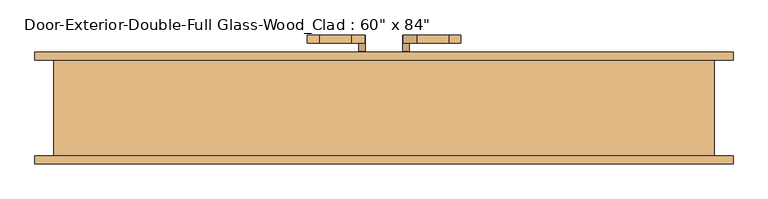
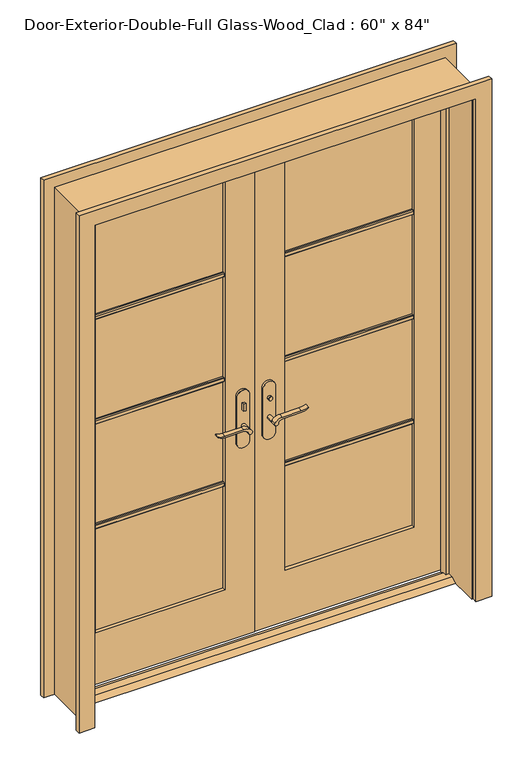
"""IFC4 building model written with IfcOpenShell, lengths in millimetres: door geometry."""

from ifc_helpers import new_model, si_unit, point, frame, frame_2d, origin, place, context, project, spatial, polyline, circle_curve, trimmed, segment, composite_curve, outline, extrude, faceted_brep, source, transform, mapped, element, save


def door_7ffae4ec(model_context):
    return source(origin(), model_context, "Body", "SolidModel", [
        extrude(outline(polyline([(19.05, 12.7), (53.975, 12.7), (79.375, 0.0), (-6.35, 0.0), (19.05, 12.7)])), frame((-762.0, 0.0, 0.0), z_axis=(1.0, 0.0, 0.0), x_axis=(0.0, 1.0, 0.0)), (0.0, 0.0, 1.0), 1524.0),
        extrude(outline(polyline([(-47.4019111, 56.2), (-57.4019111, 56.2), (-57.4019111, 66.2), (-47.4019111, 66.2), (-47.4019111, 56.2)])), frame((0.0, 0.0, 981.9), z_axis=(0.0, 0.0, 1.0), x_axis=(1.0, 0.0, 0.0)), (0.0, 0.0, 1.0), 30.0),
        extrude(outline(composite_curve([segment(trimmed(circle_curve(frame_2d((996.9, -52.4019111)), 8.0), [point((996.9, -60.4019111))], [point((996.9, -44.4019111))], False, "CARTESIAN"), True, "CONTINUOUS"), segment(trimmed(circle_curve(frame_2d((996.9, -52.4019111)), 8.0), [point((996.9, -44.4019111))], [point((996.9, -60.4019111))], False, "CARTESIAN"), True, "CONTINUOUS")], self_intersect=False)), frame((0.0, 121.125, 0.0), z_axis=(0.0, 1.0, 0.0), x_axis=(0.0, 0.0, 1.0)), (0.0, 0.0, 1.0), 10.0),
        extrude(outline(composite_curve([segment(trimmed(circle_curve(frame_2d((897.1555521, -76.0694241)), 37.2832219), [point((919.0523287, -45.8937749))], [point((934.4, -77.7693445))], False, "CARTESIAN"), True, "CONTINUOUS"), segment(polyline([(934.4, -77.7693445), (934.4, -154.045502)]), True, "CONTINUOUS"), segment(trimmed(circle_curve(frame_2d((1017.6850638, -153.9791202)), 83.2850902), [point((934.4, -154.045502))], [point((939.4, -182.4019111))], True, "CARTESIAN"), True, "CONTINUOUS"), segment(polyline([(939.4, -182.4019111), (936.6135558, -182.4019111)]), True, "CONTINUOUS"), segment(trimmed(circle_curve(frame_2d((986.6709207, -150.4622499)), 59.3791355), [point((936.6135558, -182.4019111))], [point((927.4, -154.045502))], False, "CARTESIAN"), True, "CONTINUOUS"), segment(polyline([(927.4, -154.045502), (927.4, -77.7881013)]), True, "CONTINUOUS"), segment(trimmed(circle_curve(frame_2d((909.2738613, -77.7881013)), 18.1261387), [point((927.4, -77.7881013))], [point((914.4, -60.4019111))], True, "CARTESIAN"), True, "CONTINUOUS"), segment(trimmed(circle_curve(frame_2d((914.4, -52.4019111)), 8.0), [point((914.4, -60.4019111))], [point((919.0523287, -45.8937749))], False, "CARTESIAN"), True, "CONTINUOUS")], self_intersect=False)), frame((0.0, 16.2, 0.0), z_axis=(0.0, 1.0, 0.0), x_axis=(0.0, 0.0, 1.0)), (0.0, 0.0, 1.0), 20.0),
        extrude(outline(composite_curve([segment(trimmed(circle_curve(frame_2d((914.4, -52.4019111)), 8.0), [point((914.3999903, -60.4019111))], [point((919.0523287, -45.8937749))], False, "CARTESIAN"), True, "CONTINUOUS"), segment(trimmed(circle_curve(frame_2d((897.1555521, -76.0694241)), 37.2832219), [point((919.0523287, -45.8937749))], [point((934.4, -77.7693445))], False, "CARTESIAN"), True, "CONTINUOUS"), segment(polyline([(934.4, -77.7693445), (934.4, -154.045502)]), True, "CONTINUOUS"), segment(trimmed(circle_curve(frame_2d((1017.6850638, -153.9791202)), 83.2850902), [point((934.4, -154.045502))], [point((939.4, -182.4019111))], True, "CARTESIAN"), True, "CONTINUOUS"), segment(polyline([(939.4, -182.4019111), (936.6135558, -182.4019111)]), True, "CONTINUOUS"), segment(trimmed(circle_curve(frame_2d((986.6709207, -150.4622499)), 59.3791355), [point((936.6135558, -182.4019111))], [point((927.4, -154.045502))], False, "CARTESIAN"), True, "CONTINUOUS"), segment(polyline([(927.4, -154.045502), (927.4, -77.788099)]), True, "CONTINUOUS"), segment(trimmed(circle_curve(frame_2d((909.2738682, -77.788099)), 18.1261318), [point((927.4, -77.788099))], [point((914.3999903, -60.4019111))], True, "CARTESIAN"), True, "CONTINUOUS")], self_intersect=False)), frame((0.0, 151.125, 0.0), z_axis=(0.0, 1.0, 0.0), x_axis=(0.0, 0.0, 1.0)), (0.0, 0.0, 1.0), 20.0),
        extrude(outline(composite_curve([segment(trimmed(circle_curve(frame_2d((914.4, -52.4019111)), 8.0), [point((914.4, -60.4019111))], [point((914.4, -44.4019111))], False, "CARTESIAN"), True, "CONTINUOUS"), segment(trimmed(circle_curve(frame_2d((914.4, -52.4019111)), 8.0), [point((914.4, -44.4019111))], [point((914.4, -60.4019111))], False, "CARTESIAN"), True, "CONTINUOUS")], self_intersect=False)), frame((0.0, 36.2, 0.0), z_axis=(0.0, 1.0, 0.0), x_axis=(0.0, 0.0, 1.0)), (0.0, 0.0, 1.0), 30.0),
        extrude(outline(composite_curve([segment(trimmed(circle_curve(frame_2d((914.4, -52.4019111)), 8.0), [point((914.4, -60.4019111))], [point((914.4, -44.4019111))], False, "CARTESIAN"), True, "CONTINUOUS"), segment(trimmed(circle_curve(frame_2d((914.4, -52.4019111)), 8.0), [point((914.4, -44.4019111))], [point((914.4, -60.4019111))], False, "CARTESIAN"), True, "CONTINUOUS")], self_intersect=False)), frame((0.0, 121.125, 0.0), z_axis=(0.0, 1.0, 0.0), x_axis=(0.0, 0.0, 1.0)), (0.0, 0.0, 1.0), 30.0),
        extrude(outline(composite_curve([segment(polyline([(844.4, -27.4019111), (1039.4, -27.4019111)]), True, "CONTINUOUS"), segment(trimmed(circle_curve(frame_2d((1039.4, -52.4019111)), 25.0), [point((1039.4, -27.4019111))], [point((1039.4, -77.4019111))], False, "CARTESIAN"), True, "CONTINUOUS"), segment(polyline([(1039.4, -77.4019111), (844.4, -77.4019111)]), True, "CONTINUOUS"), segment(trimmed(circle_curve(frame_2d((844.4, -52.4019111)), 25.0), [point((844.4, -77.4019111))], [point((844.4, -27.4019111))], False, "CARTESIAN"), True, "CONTINUOUS")], self_intersect=False)), frame((0.0, 66.2, 0.0), z_axis=(0.0, 1.0, 0.0), x_axis=(0.0, 0.0, 1.0)), (0.0, 0.0, 1.0), 10.0),
        extrude(outline(composite_curve([segment(polyline([(844.4, -27.4019111), (1039.4, -27.4019111)]), True, "CONTINUOUS"), segment(trimmed(circle_curve(frame_2d((1039.4, -52.4019111)), 25.0), [point((1039.4, -27.4019111))], [point((1039.4, -77.4019111))], False, "CARTESIAN"), True, "CONTINUOUS"), segment(polyline([(1039.4, -77.4019111), (844.4, -77.4019111)]), True, "CONTINUOUS"), segment(trimmed(circle_curve(frame_2d((844.4, -52.4019111)), 25.0), [point((844.4, -77.4019111))], [point((844.4, -27.4019111))], False, "CARTESIAN"), True, "CONTINUOUS")], self_intersect=False)), frame((0.0, 111.125, 0.0), z_axis=(0.0, 1.0, 0.0), x_axis=(0.0, 0.0, 1.0)), (0.0, 0.0, 1.0), 10.0),
        extrude(outline(polyline([(47.3875, 131.125), (57.3875, 131.125), (57.3875, 121.125), (47.3875, 121.125), (47.3875, 131.125)])), frame((0.0, 0.0, 981.9), z_axis=(0.0, 0.0, 1.0), x_axis=(1.0, 0.0, 0.0)), (0.0, 0.0, 1.0), 30.0),
        extrude(outline(composite_curve([segment(trimmed(circle_curve(frame_2d((996.9, 52.3875)), 8.0), [point((996.9, 60.3875))], [point((996.9, 44.3875))], False, "CARTESIAN"), True, "CONTINUOUS"), segment(trimmed(circle_curve(frame_2d((996.9, 52.3875)), 8.0), [point((996.9, 44.3875))], [point((996.9, 60.3875))], False, "CARTESIAN"), True, "CONTINUOUS")], self_intersect=False)), frame((0.0, 56.2, 0.0), z_axis=(0.0, 1.0, 0.0), x_axis=(0.0, 0.0, 1.0)), (0.0, 0.0, 1.0), 10.0),
        extrude(outline(composite_curve([segment(trimmed(circle_curve(frame_2d((914.4, 52.3875)), 8.0), [point((919.0523287, 45.8793637))], [point((914.4, 60.3875))], False, "CARTESIAN"), True, "CONTINUOUS"), segment(trimmed(circle_curve(frame_2d((909.2738613, 77.7736901)), 18.1261387), [point((914.4, 60.3875))], [point((927.4, 77.7736901))], True, "CARTESIAN"), True, "CONTINUOUS"), segment(polyline([(927.4, 77.7736901), (927.4, 154.0310909)]), True, "CONTINUOUS"), segment(trimmed(circle_curve(frame_2d((986.6709207, 150.4478388)), 59.3791355), [point((927.4, 154.0310909))], [point((936.6135558, 182.3875))], False, "CARTESIAN"), True, "CONTINUOUS"), segment(polyline([(936.6135558, 182.3875), (939.4, 182.3875)]), True, "CONTINUOUS"), segment(trimmed(circle_curve(frame_2d((1017.6850638, 153.9647091)), 83.2850902), [point((939.4, 182.3875))], [point((934.4, 154.0310909))], True, "CARTESIAN"), True, "CONTINUOUS"), segment(polyline([(934.4, 154.0310909), (934.4, 77.7549333)]), True, "CONTINUOUS"), segment(trimmed(circle_curve(frame_2d((897.1555521, 76.0550129)), 37.2832219), [point((934.4, 77.7549333))], [point((919.0523287, 45.8793637))], False, "CARTESIAN"), True, "CONTINUOUS")], self_intersect=False)), frame((0.0, 151.125, 0.0), z_axis=(0.0, 1.0, 0.0), x_axis=(0.0, 0.0, 1.0)), (0.0, 0.0, 1.0), 20.0),
        extrude(outline(composite_curve([segment(trimmed(circle_curve(frame_2d((909.2738682, 77.7736878)), 18.1261318), [point((914.3999903, 60.3875))], [point((927.4, 77.7736878))], True, "CARTESIAN"), True, "CONTINUOUS"), segment(polyline([(927.4, 77.7736878), (927.4, 154.0310909)]), True, "CONTINUOUS"), segment(trimmed(circle_curve(frame_2d((986.6709207, 150.4478388)), 59.3791355), [point((927.4, 154.0310909))], [point((936.6135558, 182.3875))], False, "CARTESIAN"), True, "CONTINUOUS"), segment(polyline([(936.6135558, 182.3875), (939.4, 182.3875)]), True, "CONTINUOUS"), segment(trimmed(circle_curve(frame_2d((1017.6850638, 153.9647091)), 83.2850902), [point((939.4, 182.3875))], [point((934.4, 154.0310909))], True, "CARTESIAN"), True, "CONTINUOUS"), segment(polyline([(934.4, 154.0310909), (934.4, 77.7549333)]), True, "CONTINUOUS"), segment(trimmed(circle_curve(frame_2d((897.1555521, 76.0550129)), 37.2832219), [point((934.4, 77.7549333))], [point((919.0523287, 45.8793637))], False, "CARTESIAN"), True, "CONTINUOUS"), segment(trimmed(circle_curve(frame_2d((914.4, 52.3875)), 8.0), [point((919.0523287, 45.8793637))], [point((914.3999903, 60.3875))], False, "CARTESIAN"), True, "CONTINUOUS")], self_intersect=False)), frame((0.0, 16.2, 0.0), z_axis=(0.0, 1.0, 0.0), x_axis=(0.0, 0.0, 1.0)), (0.0, 0.0, 1.0), 20.0),
        extrude(outline(composite_curve([segment(trimmed(circle_curve(frame_2d((914.4, 52.3875)), 8.0), [point((914.4, 60.3875))], [point((914.4, 44.3875))], False, "CARTESIAN"), True, "CONTINUOUS"), segment(trimmed(circle_curve(frame_2d((914.4, 52.3875)), 8.0), [point((914.4, 44.3875))], [point((914.4, 60.3875))], False, "CARTESIAN"), True, "CONTINUOUS")], self_intersect=False)), frame((0.0, 121.125, 0.0), z_axis=(0.0, 1.0, 0.0), x_axis=(0.0, 0.0, 1.0)), (0.0, 0.0, 1.0), 30.0),
        extrude(outline(composite_curve([segment(trimmed(circle_curve(frame_2d((914.4, 52.3875)), 8.0), [point((914.4, 60.3875))], [point((914.4, 44.3875))], False, "CARTESIAN"), True, "CONTINUOUS"), segment(trimmed(circle_curve(frame_2d((914.4, 52.3875)), 8.0), [point((914.4, 44.3875))], [point((914.4, 60.3875))], False, "CARTESIAN"), True, "CONTINUOUS")], self_intersect=False)), frame((0.0, 36.2, 0.0), z_axis=(0.0, 1.0, 0.0), x_axis=(0.0, 0.0, 1.0)), (0.0, 0.0, 1.0), 30.0),
        extrude(outline(composite_curve([segment(trimmed(circle_curve(frame_2d((844.4, 52.3875)), 25.0), [point((844.4, 27.3875))], [point((844.4, 77.3875))], False, "CARTESIAN"), True, "CONTINUOUS"), segment(polyline([(844.4, 77.3875), (1039.4, 77.3875)]), True, "CONTINUOUS"), segment(trimmed(circle_curve(frame_2d((1039.4, 52.3875)), 25.0), [point((1039.4, 77.3875))], [point((1039.4, 27.3875))], False, "CARTESIAN"), True, "CONTINUOUS"), segment(polyline([(1039.4, 27.3875), (844.4, 27.3875)]), True, "CONTINUOUS")], self_intersect=False)), frame((0.0, 111.125, 0.0), z_axis=(0.0, 1.0, 0.0), x_axis=(0.0, 0.0, 1.0)), (0.0, 0.0, 1.0), 10.0),
        extrude(outline(composite_curve([segment(trimmed(circle_curve(frame_2d((844.4, 52.3875)), 25.0), [point((844.4, 27.3875))], [point((844.4, 77.3875))], False, "CARTESIAN"), True, "CONTINUOUS"), segment(polyline([(844.4, 77.3875), (1039.4, 77.3875)]), True, "CONTINUOUS"), segment(trimmed(circle_curve(frame_2d((1039.4, 52.3875)), 25.0), [point((1039.4, 77.3875))], [point((1039.4, 27.3875))], False, "CARTESIAN"), True, "CONTINUOUS"), segment(polyline([(1039.4, 27.3875), (844.4, 27.3875)]), True, "CONTINUOUS")], self_intersect=False)), frame((0.0, 66.2, 0.0), z_axis=(0.0, 1.0, 0.0), x_axis=(0.0, 0.0, 1.0)), (0.0, 0.0, 1.0), 10.0),
        extrude(outline(polyline([(90.17, 1578.371875), (90.17, 1559.321875), (83.82, 1559.321875), (80.645, 1562.496875), (80.645, 1575.196875), (83.82, 1578.371875), (90.17, 1578.371875)])), frame((120.65, 0.0, 0.0), z_axis=(1.0, 0.0, 0.0), x_axis=(0.0, 1.0, 0.0)), (0.0, 0.0, 1.0), 520.7),
        extrude(outline(polyline([(90.17, 1132.68125), (90.17, 1113.63125), (83.82, 1113.63125), (80.645, 1116.80625), (80.645, 1129.50625), (83.82, 1132.68125), (90.17, 1132.68125)])), frame((120.65, 0.0, 0.0), z_axis=(1.0, 0.0, 0.0), x_axis=(0.0, 1.0, 0.0)), (0.0, 0.0, 1.0), 520.7),
        extrude(outline(polyline([(90.17, 686.990625), (90.17, 667.940625), (83.82, 667.940625), (80.645, 671.115625), (80.645, 683.815625), (83.82, 686.990625), (90.17, 686.990625)])), frame((120.65, 0.0, 0.0), z_axis=(1.0, 0.0, 0.0), x_axis=(0.0, 1.0, 0.0)), (0.0, 0.0, 1.0), 520.7),
        extrude(outline(polyline([(97.155, 1578.371875), (103.505, 1578.371875), (106.68, 1575.196875), (106.68, 1562.496875), (103.505, 1559.321875), (97.155, 1559.321875), (97.155, 1578.371875)])), frame((-641.35, 0.0, 0.0), z_axis=(1.0, 0.0, 0.0), x_axis=(0.0, 1.0, 0.0)), (0.0, 0.0, 1.0), 520.7),
        extrude(outline(polyline([(97.155, 1132.68125), (103.505, 1132.68125), (106.68, 1129.50625), (106.68, 1116.80625), (103.505, 1113.63125), (97.155, 1113.63125), (97.155, 1132.68125)])), frame((-641.35, 0.0, 0.0), z_axis=(1.0, 0.0, 0.0), x_axis=(0.0, 1.0, 0.0)), (0.0, 0.0, 1.0), 520.7),
        extrude(outline(polyline([(97.155, 686.990625), (103.505, 686.990625), (106.68, 683.815625), (106.68, 671.115625), (103.505, 667.940625), (97.155, 667.940625), (97.155, 686.990625)])), frame((-641.35, 0.0, 0.0), z_axis=(1.0, 0.0, 0.0), x_axis=(0.0, 1.0, 0.0)), (0.0, 0.0, 1.0), 520.7),
        extrude(outline(polyline([(97.155, 1578.371875), (103.505, 1578.371875), (106.68, 1575.196875), (106.68, 1562.496875), (103.505, 1559.321875), (97.155, 1559.321875), (97.155, 1578.371875)])), frame((120.65, 0.0, 0.0), z_axis=(1.0, 0.0, 0.0), x_axis=(0.0, 1.0, 0.0)), (0.0, 0.0, 1.0), 520.7),
        extrude(outline(polyline([(97.155, 1132.68125), (103.505, 1132.68125), (106.68, 1129.50625), (106.68, 1116.80625), (103.505, 1113.63125), (97.155, 1113.63125), (97.155, 1132.68125)])), frame((120.65, 0.0, 0.0), z_axis=(1.0, 0.0, 0.0), x_axis=(0.0, 1.0, 0.0)), (0.0, 0.0, 1.0), 520.7),
        extrude(outline(polyline([(97.155, 686.990625), (103.505, 686.990625), (106.68, 683.815625), (106.68, 671.115625), (103.505, 667.940625), (97.155, 667.940625), (97.155, 686.990625)])), frame((120.65, 0.0, 0.0), z_axis=(1.0, 0.0, 0.0), x_axis=(0.0, 1.0, 0.0)), (0.0, 0.0, 1.0), 520.7),
        extrude(outline(polyline([(90.17, 1578.371875), (90.17, 1559.321875), (83.82, 1559.321875), (80.645, 1562.496875), (80.645, 1575.196875), (83.82, 1578.371875), (90.17, 1578.371875)])), frame((-641.35, 0.0, 0.0), z_axis=(1.0, 0.0, 0.0), x_axis=(0.0, 1.0, 0.0)), (0.0, 0.0, 1.0), 520.7),
        extrude(outline(polyline([(90.17, 1132.68125), (90.17, 1113.63125), (83.82, 1113.63125), (80.645, 1116.80625), (80.645, 1129.50625), (83.82, 1132.68125), (90.17, 1132.68125)])), frame((-641.35, 0.0, 0.0), z_axis=(1.0, 0.0, 0.0), x_axis=(0.0, 1.0, 0.0)), (0.0, 0.0, 1.0), 520.7),
        extrude(outline(polyline([(90.17, 686.990625), (90.17, 667.940625), (83.82, 667.940625), (80.645, 671.115625), (80.645, 683.815625), (83.82, 686.990625), (90.17, 686.990625)])), frame((-641.35, 0.0, 0.0), z_axis=(1.0, 0.0, 0.0), x_axis=(0.0, 1.0, 0.0)), (0.0, 0.0, 1.0), 520.7),
        extrude(outline(polyline([(0.0, 768.35), (0.0, 831.85), (2203.45, 831.85), (2203.45, -831.85), (0.0, -831.85), (0.0, -768.35), (2139.95, -768.35), (2139.95, 768.35), (0.0, 768.35)])), frame((0.0, -136.525, 0.0), z_axis=(0.0, 1.0, 0.0), x_axis=(0.0, 0.0, 1.0)), (0.0, 0.0, 1.0), 19.05),
        extrude(outline(polyline([(0.0, 768.35), (0.0, 831.85), (2203.45, 831.85), (2203.45, -831.85), (0.0, -831.85), (0.0, -768.35), (2139.95, -768.35), (2139.95, 768.35), (0.0, 768.35)])), frame((0.0, 111.125, 0.0), z_axis=(0.0, 1.0, 0.0), x_axis=(0.0, 0.0, 1.0)), (0.0, 0.0, 1.0), 19.05),
        faceted_brep([(787.4, 111.125, 0.0), (787.4, -117.475, 0.0), (762.0, -117.475, 0.0), (762.0, 41.275, 0.0), (749.3, 41.275, 0.0), (749.3, 76.2, 0.0), (762.0, 76.2, 0.0), (762.0, 111.125, 0.0), (787.4, 111.125, 2159.0), (787.4, -117.475, 2159.0), (-787.4, -117.475, 2159.0), (-787.4, -117.475, 0.0), (-762.0, -117.475, 0.0), (-762.0, -117.475, 2133.6), (762.0, -117.475, 2133.6), (762.0, 41.275, 2133.6), (-762.0, 41.275, 2133.6), (-762.0, 41.275, 0.0), (-749.3, 41.275, 0.0), (-749.3, 41.275, 2120.9), (749.3, 41.275, 2120.9), (749.3, 76.2, 2120.9), (1.5875, 76.2, 2120.9), (-1.6019111, 76.2, 2120.9), (-749.3, 76.2, 2120.9), (-749.3, 76.2, 0.0), (-762.0, 76.2, 0.0), (-762.0, 76.2, 2133.6), (-1.6019111, 76.2, 2133.6), (1.5875, 76.2, 2133.6), (762.0, 76.2, 2133.6), (762.0, 111.125, 2133.6), (1.5875, 111.125, 2133.6), (-1.6019111, 111.125, 2133.6), (-762.0, 111.125, 2133.6), (-762.0, 111.125, 0.0), (-787.4, 111.125, 0.0), (-787.4, 111.125, 2159.0)], [[[0, 1, 2, 3, 4, 5, 6, 7]], [[1, 0, 8, 9]], [[2, 1, 9, 10, 11, 12, 13, 14]], [[3, 2, 14, 15]], [[4, 3, 15, 16, 17, 18, 19, 20]], [[5, 4, 20, 21]], [[6, 5, 21, 22, 23, 24, 25, 26, 27, 28, 29, 30]], [[7, 6, 30, 31]], [[0, 7, 31, 32, 33, 34, 35, 36, 37, 8]], [[9, 8, 37, 10]], [[14, 13, 16, 15]], [[20, 19, 24, 23, 22, 21]], [[31, 30, 29, 28, 27, 34, 33, 32]], [[12, 11, 36, 35, 26, 25, 18, 17]], [[11, 10, 37, 36]], [[13, 12, 17, 16]], [[19, 18, 25, 24]], [[27, 26, 35, 34]]]),
        extrude(outline(polyline([(12.7, 762.0), (2133.6, 762.0), (2133.6, 1.5875), (12.7, 1.5875), (12.7, 762.0)]), holes=[polyline([(2014.5375, 120.65), (2014.5375, 641.35), (231.775, 641.35), (231.775, 120.65), (2014.5375, 120.65)])]), frame((0.0, 76.2, 0.0), z_axis=(0.0, 1.0, 0.0), x_axis=(0.0, 0.0, 1.0)), (0.0, 0.0, 1.0), 34.925),
        extrude(outline(polyline([(2133.6, -762.0), (12.7, -762.0), (12.7, -1.6019111), (2133.6, -1.6019111), (2133.6, -762.0)]), holes=[polyline([(231.775, -641.35), (2014.5375, -641.35), (2014.5375, -120.65), (231.775, -120.65), (231.775, -641.35)])]), frame((0.0, 76.2, 0.0), z_axis=(0.0, 1.0, 0.0), x_axis=(0.0, 0.0, 1.0)), (0.0, 0.0, 1.0), 34.925),
        extrude(outline(polyline([(641.35, 90.17), (120.65, 90.17), (120.65, 97.155), (641.35, 97.155), (641.35, 90.17)])), frame((0.0, 0.0, 231.775), z_axis=(0.0, 0.0, 1.0), x_axis=(1.0, 0.0, 0.0)), (0.0, 0.0, 1.0), 1782.7625),
        extrude(outline(polyline([(-120.65, 90.17), (-641.35, 90.17), (-641.35, 97.155), (-120.65, 97.155), (-120.65, 90.17)])), frame((0.0, 0.0, 231.775), z_axis=(0.0, 0.0, 1.0), x_axis=(1.0, 0.0, 0.0)), (0.0, 0.0, 1.0), 1782.7625),
    ])


if __name__ == "__main__":
    model = new_model("IFC4")
    model_context = context("Model", 3, world=origin())
    ifc_project = project(units=[si_unit("LENGTHUNIT", "METRE", prefix="MILLI")], contexts=[model_context])
    site = spatial("IfcSite", under=ifc_project)
    building = spatial("IfcBuilding", under=site)
    placement = place(None, origin())
    door_shape = door_7ffae4ec(model_context)
    element("IfcDoor", 1, ObjectType="Door-Exterior-Double-Full Glass-Wood_Clad : 60\" x 84\"", at=placement, inside=building, context=model_context, shape_type="MappedRepresentation", body=[
        mapped(door_shape, transform((0.0, 0.0, 0.0), x_axis=(1.0, 0.0, 0.0), y_axis=(0.0, 1.0, 0.0), z_axis=(0.0, 0.0, 1.0))),
    ])
    save(model, "model.ifc")

# Revit data of these elements
# Type "Door-Exterior-Double-Full Glass-Wood_Clad : 60\" x 84\""
#   Type Mark = "12"
#   Assembly Code = "B2030100"
#   Analytic Construction = "French door, wood frame with double glass"
#   Top Rail = 0' - 4 11/16"
#   Threshold Offset [instance default] = 0' - 0 1/2"
#   Thickness = 0' - 1 3/8"
#   Thermal Resistance (R) = 1.9158 (h·ft²·°F)/BTU
#   Swing Angle [instance default] = 90.00°
#   Stiles = 0' - 4 3/4"
#   Rough Width = 5' - 2"
#   Rough Height = 7' - 1"
#   Panel Width = 2' - 6"
#   Door Offset [instance default] = 0' - 0"
#   Height = 7' - 0"
#   Width = 5' - 0"
#   Heat Transfer Coefficient (U) = 0.5220 BTU/(h·ft²·°F)
#   Bottom Rail = 0' - 9 1/8"
#   Exterior Trim [instance default] = yes
#   Threshold [instance default] = yes
#   Show Grill [instance default] = yes
#   Function = 1
#   Trim Material = Cherry
#   Threshold Material = Cherry
#   Panel Material = Cherry
#   Glazing = Glass
#   Frame Material = Cherry
#   Door Handle Material = Aluminum
#   Visual Light Transmittance = 0
#   Solar Heat Gain Coefficient = 0
#   Wall Closure = (empty or 0)
#   Construction Type = (empty or 0)
# Element 1 (IfcDoor, "Door-Exterior-Double-Full Glass-Wood_Clad : 60\" x 84\"")
#   Materials on its faces: "Cherry", "Aluminum", "Glass"
# Materials
#   "Cherry": class "Wood", colour RGB 226 177 128, transparency 0, Description = "Prunus Serotina", Cost = 0
#   "Glass": class "Glass", colour RGB 0 128 192, transparency 0.75, Description = "Soda Lime Glass", Cost = 0
#   "Aluminum": class "Metal", colour RGB 247 247 247, transparency 0, Description = "Aluminum 6061", Cost = 0
